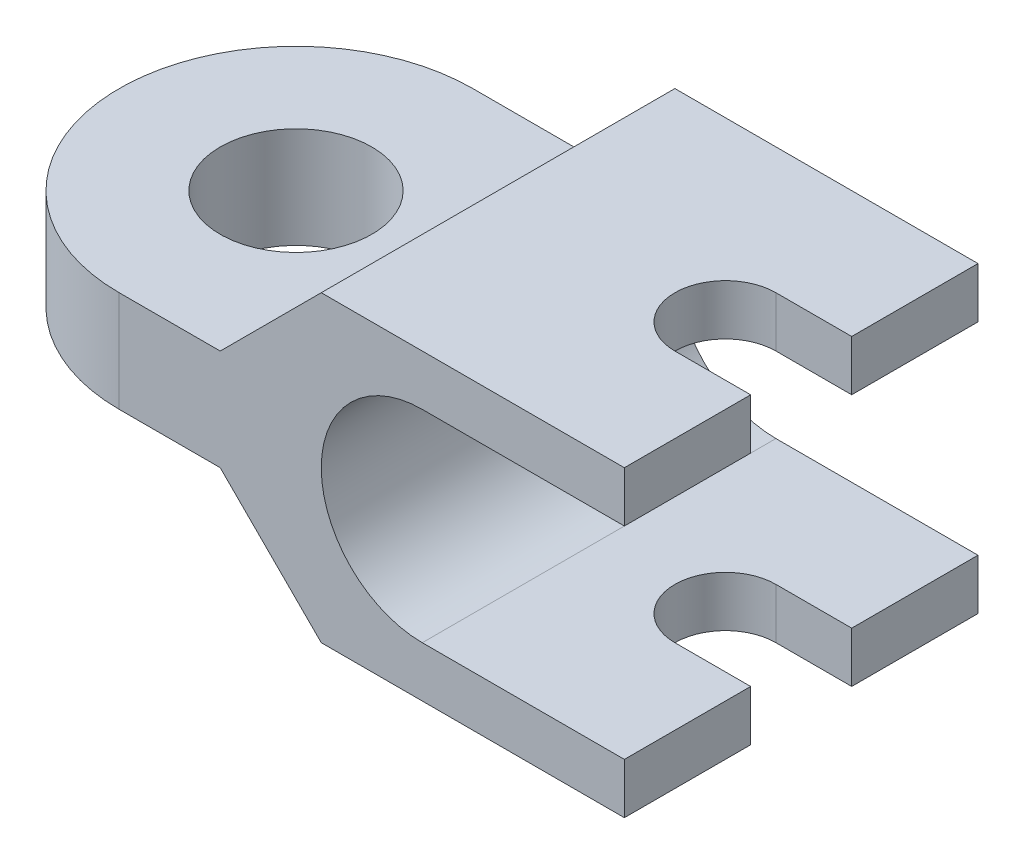
ISO-10303-21;
HEADER;
FILE_DESCRIPTION(('STEP AP214'),'2;1');
FILE_NAME('part.step','',(''),(''),'','','');
FILE_SCHEMA(('AUTOMOTIVE_DESIGN { 1 0 10303 214 1 1 1 1 }'));
ENDSEC;
DATA;
#1=APPLICATION_CONTEXT('core data for automotive mechanical design processes');
#2=APPLICATION_PROTOCOL_DEFINITION('international standard','automotive_design',2000,#1);
#3=PRODUCT_CONTEXT('',#1,'mechanical');
#4=PRODUCT('Part','Part','',(#3));
#5=PRODUCT_RELATED_PRODUCT_CATEGORY('part','',(#4));
#6=PRODUCT_DEFINITION_FORMATION('','',#4);
#7=PRODUCT_DEFINITION_CONTEXT('part definition',#1,'design');
#8=PRODUCT_DEFINITION('design','',#6,#7);
#9=PRODUCT_DEFINITION_SHAPE('','',#8);
#10=(LENGTH_UNIT() NAMED_UNIT(*) SI_UNIT(.MILLI.,.METRE.));
#11=(NAMED_UNIT(*) PLANE_ANGLE_UNIT() SI_UNIT($,.RADIAN.));
#12=(NAMED_UNIT(*) SI_UNIT($,.STERADIAN.) SOLID_ANGLE_UNIT());
#13=UNCERTAINTY_MEASURE_WITH_UNIT(LENGTH_MEASURE(1.E-05),#10,'distance_accuracy_value','');
#14=(GEOMETRIC_REPRESENTATION_CONTEXT(3) GLOBAL_UNCERTAINTY_ASSIGNED_CONTEXT((#13)) GLOBAL_UNIT_ASSIGNED_CONTEXT((#10,
#11,#12)) REPRESENTATION_CONTEXT('',''));
#15=CARTESIAN_POINT('',(0.,0.,0.));
#16=DIRECTION('',(0.,0.,1.));
#17=DIRECTION('',(1.,0.,0.));
#18=AXIS2_PLACEMENT_3D('',#15,#16,#17);
#19=CARTESIAN_POINT('',(-40.,-9.99999999999998,35.));
#20=DIRECTION('',(0.707106781186548,0.707106781186547,0.));
#21=DIRECTION('',(-0.707106781186547,0.707106781186548,0.));
#22=AXIS2_PLACEMENT_3D('',#19,#20,#21);
#23=PLANE('',#22);
#24=DIRECTION('',(-0.707106781186547,0.707106781186548,0.));
#25=VECTOR('',#24,1.);
#26=CARTESIAN_POINT('',(-30.,-20.,15.));
#27=LINE('',#26,#25);
#28=CARTESIAN_POINT('',(-30.,-20.,15.));
#29=VERTEX_POINT('',#28);
#30=CARTESIAN_POINT('',(-40.,-9.99999999999998,15.));
#31=VERTEX_POINT('',#30);
#32=EDGE_CURVE('E239',#29,#31,#27,.T.);
#33=ORIENTED_EDGE('',*,*,#32,.F.);
#34=DIRECTION('',(0.,0.,1.));
#35=VECTOR('',#34,1.);
#36=CARTESIAN_POINT('',(-30.,-20.,-15.));
#37=LINE('',#36,#35);
#38=CARTESIAN_POINT('',(-30.,-20.,-15.));
#39=VERTEX_POINT('',#38);
#40=EDGE_CURVE('E221',#39,#29,#37,.T.);
#41=ORIENTED_EDGE('',*,*,#40,.F.);
#42=DIRECTION('',(-0.707106781186547,0.707106781186548,0.));
#43=VECTOR('',#42,1.);
#44=CARTESIAN_POINT('',(-30.,-20.,-15.));
#45=LINE('',#44,#43);
#46=CARTESIAN_POINT('',(-40.,-9.99999999999998,-15.));
#47=VERTEX_POINT('',#46);
#48=EDGE_CURVE('E60',#39,#47,#45,.T.);
#49=ORIENTED_EDGE('',*,*,#48,.T.);
#50=DIRECTION('',(0.,0.,-1.));
#51=VECTOR('',#50,1.);
#52=CARTESIAN_POINT('',(-40.,-9.99999999999998,35.));
#53=LINE('',#52,#51);
#54=CARTESIAN_POINT('',(-40.,-9.99999999999998,-35.));
#55=VERTEX_POINT('',#54);
#56=EDGE_CURVE('E224',#47,#55,#53,.T.);
#57=ORIENTED_EDGE('',*,*,#56,.T.);
#58=DIRECTION('',(0.707106781186547,-0.707106781186548,0.));
#59=VECTOR('',#58,1.);
#60=CARTESIAN_POINT('',(-40.,-9.99999999999998,-35.));
#61=LINE('',#60,#59);
#62=CARTESIAN_POINT('',(-20.,-30.,-35.));
#63=VERTEX_POINT('',#62);
#64=EDGE_CURVE('E361',#55,#63,#61,.T.);
#65=ORIENTED_EDGE('',*,*,#64,.T.);
#66=DIRECTION('',(0.,0.,-1.));
#67=VECTOR('',#66,1.);
#68=CARTESIAN_POINT('',(-20.,-30.,35.));
#69=LINE('',#68,#67);
#70=CARTESIAN_POINT('',(-20.,-30.,35.));
#71=VERTEX_POINT('',#70);
#72=EDGE_CURVE('E367',#71,#63,#69,.T.);
#73=ORIENTED_EDGE('',*,*,#72,.F.);
#74=DIRECTION('',(0.707106781186547,-0.707106781186548,0.));
#75=VECTOR('',#74,1.);
#76=CARTESIAN_POINT('',(-40.,-9.99999999999998,35.));
#77=LINE('',#76,#75);
#78=CARTESIAN_POINT('',(-40.,-9.99999999999998,35.));
#79=VERTEX_POINT('',#78);
#80=EDGE_CURVE('E338',#79,#71,#77,.T.);
#81=ORIENTED_EDGE('',*,*,#80,.F.);
#82=EDGE_CURVE('E373',#79,#31,#53,.T.);
#83=ORIENTED_EDGE('',*,*,#82,.T.);
#84=EDGE_LOOP('',(#33,#41,#49,#57,#65,#73,#81,#83));
#85=FACE_BOUND('',#84,.T.);
#86=ADVANCED_FACE('F41',(#85),#23,.F.);
#87=CARTESIAN_POINT('',(40.,-30.,35.));
#88=DIRECTION('',(-1.,0.,0.));
#89=DIRECTION('',(0.,0.,1.));
#90=AXIS2_PLACEMENT_3D('',#87,#88,#89);
#91=PLANE('',#90);
#92=DIRECTION('',(0.,1.,0.));
#93=VECTOR('',#92,1.);
#94=CARTESIAN_POINT('',(40.,-30.,-10.));
#95=LINE('',#94,#93);
#96=CARTESIAN_POINT('',(40.,-30.,-10.));
#97=VERTEX_POINT('',#96);
#98=CARTESIAN_POINT('',(40.,-20.,-10.));
#99=VERTEX_POINT('',#98);
#100=EDGE_CURVE('E301',#97,#99,#95,.T.);
#101=ORIENTED_EDGE('',*,*,#100,.F.);
#102=DIRECTION('',(0.,0.,-1.));
#103=VECTOR('',#102,1.);
#104=CARTESIAN_POINT('',(40.,-30.,35.));
#105=LINE('',#104,#103);
#106=CARTESIAN_POINT('',(40.,-30.,-35.));
#107=VERTEX_POINT('',#106);
#108=EDGE_CURVE('E336',#97,#107,#105,.T.);
#109=ORIENTED_EDGE('',*,*,#108,.T.);
#110=DIRECTION('',(0.,1.,0.));
#111=VECTOR('',#110,1.);
#112=CARTESIAN_POINT('',(40.,-30.,-35.));
#113=LINE('',#112,#111);
#114=CARTESIAN_POINT('',(40.,-20.,-35.));
#115=VERTEX_POINT('',#114);
#116=EDGE_CURVE('E314',#107,#115,#113,.T.);
#117=ORIENTED_EDGE('',*,*,#116,.T.);
#118=DIRECTION('',(0.,0.,-1.));
#119=VECTOR('',#118,1.);
#120=CARTESIAN_POINT('',(40.,-20.,35.));
#121=LINE('',#120,#119);
#122=EDGE_CURVE('E400',#99,#115,#121,.T.);
#123=ORIENTED_EDGE('',*,*,#122,.F.);
#124=EDGE_LOOP('',(#101,#109,#117,#123));
#125=FACE_BOUND('',#124,.T.);
#126=ADVANCED_FACE('F500',(#125),#91,.F.);
#127=CARTESIAN_POINT('',(40.,20.,35.));
#128=DIRECTION('',(-1.,0.,0.));
#129=DIRECTION('',(0.,0.,1.));
#130=AXIS2_PLACEMENT_3D('',#127,#128,#129);
#131=PLANE('',#130);
#132=CARTESIAN_POINT('',(40.,20.,-10.));
#133=VERTEX_POINT('',#132);
#134=CARTESIAN_POINT('',(40.,30.,-10.));
#135=VERTEX_POINT('',#134);
#136=EDGE_CURVE('E290',#133,#135,#95,.T.);
#137=ORIENTED_EDGE('',*,*,#136,.F.);
#138=DIRECTION('',(0.,0.,-1.));
#139=VECTOR('',#138,1.);
#140=CARTESIAN_POINT('',(40.,20.,35.));
#141=LINE('',#140,#139);
#142=CARTESIAN_POINT('',(40.,20.,-35.));
#143=VERTEX_POINT('',#142);
#144=EDGE_CURVE('E390',#133,#143,#141,.T.);
#145=ORIENTED_EDGE('',*,*,#144,.T.);
#146=DIRECTION('',(0.,1.,0.));
#147=VECTOR('',#146,1.);
#148=CARTESIAN_POINT('',(40.,20.,-35.));
#149=LINE('',#148,#147);
#150=CARTESIAN_POINT('',(40.,30.,-35.));
#151=VERTEX_POINT('',#150);
#152=EDGE_CURVE('E348',#143,#151,#149,.T.);
#153=ORIENTED_EDGE('',*,*,#152,.T.);
#154=DIRECTION('',(0.,0.,-1.));
#155=VECTOR('',#154,1.);
#156=CARTESIAN_POINT('',(40.,30.,35.));
#157=LINE('',#156,#155);
#158=EDGE_CURVE('E382',#135,#151,#157,.T.);
#159=ORIENTED_EDGE('',*,*,#158,.F.);
#160=EDGE_LOOP('',(#137,#145,#153,#159));
#161=FACE_BOUND('',#160,.T.);
#162=ADVANCED_FACE('F425',(#161),#131,.F.);
#163=CARTESIAN_POINT('',(40.,30.,35.));
#164=DIRECTION('',(0.,-1.,0.));
#165=DIRECTION('',(0.,0.,-1.));
#166=AXIS2_PLACEMENT_3D('',#163,#164,#165);
#167=PLANE('',#166);
#168=DIRECTION('',(-1.,0.,0.));
#169=VECTOR('',#168,1.);
#170=CARTESIAN_POINT('',(40.,30.,-10.));
#171=LINE('',#170,#169);
#172=CARTESIAN_POINT('',(25.,30.,-10.));
#173=VERTEX_POINT('',#172);
#174=EDGE_CURVE('E269',#135,#173,#171,.T.);
#175=ORIENTED_EDGE('',*,*,#174,.F.);
#176=ORIENTED_EDGE('',*,*,#158,.T.);
#177=DIRECTION('',(-1.,0.,0.));
#178=VECTOR('',#177,1.);
#179=CARTESIAN_POINT('',(40.,30.,-35.));
#180=LINE('',#179,#178);
#181=CARTESIAN_POINT('',(-20.,30.,-35.));
#182=VERTEX_POINT('',#181);
#183=EDGE_CURVE('E352',#151,#182,#180,.T.);
#184=ORIENTED_EDGE('',*,*,#183,.T.);
#185=DIRECTION('',(0.,0.,-1.));
#186=VECTOR('',#185,1.);
#187=CARTESIAN_POINT('',(-20.,30.,35.));
#188=LINE('',#187,#186);
#189=CARTESIAN_POINT('',(-20.,30.,35.));
#190=VERTEX_POINT('',#189);
#191=EDGE_CURVE('E379',#190,#182,#188,.T.);
#192=ORIENTED_EDGE('',*,*,#191,.F.);
#193=DIRECTION('',(-1.,0.,0.));
#194=VECTOR('',#193,1.);
#195=CARTESIAN_POINT('',(40.,30.,35.));
#196=LINE('',#195,#194);
#197=CARTESIAN_POINT('',(40.,30.,35.));
#198=VERTEX_POINT('',#197);
#199=EDGE_CURVE('E330',#198,#190,#196,.T.);
#200=ORIENTED_EDGE('',*,*,#199,.F.);
#201=CARTESIAN_POINT('',(40.,30.,10.));
#202=VERTEX_POINT('',#201);
#203=EDGE_CURVE('E383',#198,#202,#157,.T.);
#204=ORIENTED_EDGE('',*,*,#203,.T.);
#205=DIRECTION('',(1.,0.,0.));
#206=VECTOR('',#205,1.);
#207=CARTESIAN_POINT('',(25.,30.,10.));
#208=LINE('',#207,#206);
#209=CARTESIAN_POINT('',(25.,30.,9.99999999999999));
#210=VERTEX_POINT('',#209);
#211=EDGE_CURVE('E277',#210,#202,#208,.T.);
#212=ORIENTED_EDGE('',*,*,#211,.F.);
#213=CARTESIAN_POINT('',(25.,30.,0.));
#214=DIRECTION('',(0.,1.,0.));
#215=DIRECTION('',(0.,0.,1.));
#216=AXIS2_PLACEMENT_3D('',#213,#214,#215);
#217=CIRCLE('',#216,10.);
#218=EDGE_CURVE('E272',#173,#210,#217,.T.);
#219=ORIENTED_EDGE('',*,*,#218,.F.);
#220=EDGE_LOOP('',(#175,#176,#184,#192,#200,#204,#212,#219));
#221=FACE_BOUND('',#220,.T.);
#222=ADVANCED_FACE('F426',(#221),#167,.F.);
#223=CARTESIAN_POINT('',(-60.,9.99999999999998,0.));
#224=DIRECTION('',(0.,-1.,0.));
#225=DIRECTION('',(0.,0.,-1.));
#226=AXIS2_PLACEMENT_3D('',#223,#224,#225);
#227=CYLINDRICAL_SURFACE('',#226,35.);
#228=DIRECTION('',(0.,-1.,0.));
#229=VECTOR('',#228,1.);
#230=CARTESIAN_POINT('',(-60.,0.,35.));
#231=LINE('',#230,#229);
#232=CARTESIAN_POINT('',(-60.,9.99999999999998,35.));
#233=VERTEX_POINT('',#232);
#234=CARTESIAN_POINT('',(-60.,-9.99999999999998,35.));
#235=VERTEX_POINT('',#234);
#236=EDGE_CURVE('E402',#233,#235,#231,.T.);
#237=ORIENTED_EDGE('',*,*,#236,.F.);
#238=CARTESIAN_POINT('',(-60.,9.99999999999998,0.));
#239=DIRECTION('',(0.,-1.,0.));
#240=DIRECTION('',(1.,0.,0.));
#241=AXIS2_PLACEMENT_3D('',#238,#239,#240);
#242=CIRCLE('',#241,35.);
#243=CARTESIAN_POINT('',(-60.,9.99999999999998,-35.));
#244=VERTEX_POINT('',#243);
#245=EDGE_CURVE('E409',#244,#233,#242,.F.);
#246=ORIENTED_EDGE('',*,*,#245,.F.);
#247=DIRECTION('',(0.,1.,0.));
#248=VECTOR('',#247,1.);
#249=CARTESIAN_POINT('',(-60.,9.99999999999998,-35.));
#250=LINE('',#249,#248);
#251=CARTESIAN_POINT('',(-60.,-9.99999999999998,-35.));
#252=VERTEX_POINT('',#251);
#253=EDGE_CURVE('E404',#252,#244,#250,.T.);
#254=ORIENTED_EDGE('',*,*,#253,.F.);
#255=CARTESIAN_POINT('',(-60.,-9.99999999999998,0.));
#256=DIRECTION('',(0.,1.,0.));
#257=DIRECTION('',(-1.,0.,0.));
#258=AXIS2_PLACEMENT_3D('',#255,#256,#257);
#259=CIRCLE('',#258,35.);
#260=EDGE_CURVE('E410',#235,#252,#259,.F.);
#261=ORIENTED_EDGE('',*,*,#260,.F.);
#262=EDGE_LOOP('',(#237,#246,#254,#261));
#263=FACE_BOUND('',#262,.T.);
#264=ADVANCED_FACE('F42',(#263),#227,.T.);
#265=CARTESIAN_POINT('',(40.,-30.,35.));
#266=VERTEX_POINT('',#265);
#267=CARTESIAN_POINT('',(40.,-30.,10.));
#268=VERTEX_POINT('',#267);
#269=EDGE_CURVE('E370',#266,#268,#105,.T.);
#270=ORIENTED_EDGE('',*,*,#269,.T.);
#271=DIRECTION('',(0.,1.,0.));
#272=VECTOR('',#271,1.);
#273=CARTESIAN_POINT('',(40.,-30.,10.));
#274=LINE('',#273,#272);
#275=CARTESIAN_POINT('',(40.,-20.,10.));
#276=VERTEX_POINT('',#275);
#277=EDGE_CURVE('E287',#268,#276,#274,.T.);
#278=ORIENTED_EDGE('',*,*,#277,.T.);
#279=CARTESIAN_POINT('',(40.,-20.,35.));
#280=VERTEX_POINT('',#279);
#281=EDGE_CURVE('E397',#280,#276,#121,.T.);
#282=ORIENTED_EDGE('',*,*,#281,.F.);
#283=DIRECTION('',(0.,1.,0.));
#284=VECTOR('',#283,1.);
#285=CARTESIAN_POINT('',(40.,-30.,35.));
#286=LINE('',#285,#284);
#287=EDGE_CURVE('E312',#266,#280,#286,.T.);
#288=ORIENTED_EDGE('',*,*,#287,.F.);
#289=EDGE_LOOP('',(#270,#278,#282,#288));
#290=FACE_BOUND('',#289,.T.);
#291=ADVANCED_FACE('F485',(#290),#91,.F.);
#292=CARTESIAN_POINT('',(40.,-20.,35.));
#293=DIRECTION('',(0.,-1.,0.));
#294=DIRECTION('',(1.,0.,0.));
#295=AXIS2_PLACEMENT_3D('',#292,#293,#294);
#296=PLANE('',#295);
#297=ORIENTED_EDGE('',*,*,#281,.T.);
#298=DIRECTION('',(-1.,0.,0.));
#299=VECTOR('',#298,1.);
#300=CARTESIAN_POINT('',(40.,-20.,10.));
#301=LINE('',#300,#299);
#302=CARTESIAN_POINT('',(25.,-20.,9.99999999999999));
#303=VERTEX_POINT('',#302);
#304=EDGE_CURVE('E313',#276,#303,#301,.T.);
#305=ORIENTED_EDGE('',*,*,#304,.T.);
#306=CARTESIAN_POINT('',(25.,-20.,0.));
#307=DIRECTION('',(0.,-1.,0.));
#308=DIRECTION('',(1.,0.,0.));
#309=AXIS2_PLACEMENT_3D('',#306,#307,#308);
#310=CIRCLE('',#309,10.);
#311=CARTESIAN_POINT('',(25.,-20.,-10.));
#312=VERTEX_POINT('',#311);
#313=EDGE_CURVE('E304',#303,#312,#310,.T.);
#314=ORIENTED_EDGE('',*,*,#313,.T.);
#315=DIRECTION('',(1.,0.,0.));
#316=VECTOR('',#315,1.);
#317=CARTESIAN_POINT('',(40.,-20.,-10.));
#318=LINE('',#317,#316);
#319=EDGE_CURVE('E306',#312,#99,#318,.T.);
#320=ORIENTED_EDGE('',*,*,#319,.T.);
#321=ORIENTED_EDGE('',*,*,#122,.T.);
#322=DIRECTION('',(-1.,0.,0.));
#323=VECTOR('',#322,1.);
#324=CARTESIAN_POINT('',(40.,-20.,-35.));
#325=LINE('',#324,#323);
#326=CARTESIAN_POINT('',(0.,-20.,-35.));
#327=VERTEX_POINT('',#326);
#328=EDGE_CURVE('E342',#115,#327,#325,.T.);
#329=ORIENTED_EDGE('',*,*,#328,.T.);
#330=DIRECTION('',(0.,0.,-1.));
#331=VECTOR('',#330,1.);
#332=CARTESIAN_POINT('',(0.,-20.,35.));
#333=LINE('',#332,#331);
#334=CARTESIAN_POINT('',(0.,-20.,35.));
#335=VERTEX_POINT('',#334);
#336=EDGE_CURVE('E395',#335,#327,#333,.T.);
#337=ORIENTED_EDGE('',*,*,#336,.F.);
#338=DIRECTION('',(-1.,0.,0.));
#339=VECTOR('',#338,1.);
#340=CARTESIAN_POINT('',(40.,-20.,35.));
#341=LINE('',#340,#339);
#342=EDGE_CURVE('E318',#280,#335,#341,.T.);
#343=ORIENTED_EDGE('',*,*,#342,.F.);
#344=EDGE_LOOP('',(#297,#305,#314,#320,#321,#329,#337,#343));
#345=FACE_BOUND('',#344,.T.);
#346=ADVANCED_FACE('F484',(#345),#296,.F.);
#347=CARTESIAN_POINT('',(0.,0.,35.));
#348=DIRECTION('',(0.,0.,-1.));
#349=DIRECTION('',(-1.,0.,0.));
#350=AXIS2_PLACEMENT_3D('',#347,#348,#349);
#351=CYLINDRICAL_SURFACE('',#350,20.);
#352=CARTESIAN_POINT('',(0.,0.,-35.));
#353=DIRECTION('',(0.,0.,-1.));
#354=DIRECTION('',(-1.,0.,0.));
#355=AXIS2_PLACEMENT_3D('',#352,#353,#354);
#356=CIRCLE('',#355,20.);
#357=CARTESIAN_POINT('',(0.,20.,-35.));
#358=VERTEX_POINT('',#357);
#359=EDGE_CURVE('E344',#327,#358,#356,.T.);
#360=ORIENTED_EDGE('',*,*,#359,.T.);
#361=DIRECTION('',(0.,0.,-1.));
#362=VECTOR('',#361,1.);
#363=CARTESIAN_POINT('',(0.,20.,35.));
#364=LINE('',#363,#362);
#365=CARTESIAN_POINT('',(0.,20.,35.));
#366=VERTEX_POINT('',#365);
#367=EDGE_CURVE('E393',#366,#358,#364,.T.);
#368=ORIENTED_EDGE('',*,*,#367,.F.);
#369=CARTESIAN_POINT('',(0.,0.,35.));
#370=DIRECTION('',(0.,0.,-1.));
#371=DIRECTION('',(-1.,0.,0.));
#372=AXIS2_PLACEMENT_3D('',#369,#370,#371);
#373=CIRCLE('',#372,20.);
#374=EDGE_CURVE('E321',#335,#366,#373,.T.);
#375=ORIENTED_EDGE('',*,*,#374,.F.);
#376=ORIENTED_EDGE('',*,*,#336,.T.);
#377=EDGE_LOOP('',(#360,#368,#375,#376));
#378=FACE_BOUND('',#377,.T.);
#379=ADVANCED_FACE('F486',(#378),#351,.F.);
#380=CARTESIAN_POINT('',(0.,20.,35.));
#381=DIRECTION('',(0.,1.,0.));
#382=DIRECTION('',(-1.,0.,0.));
#383=AXIS2_PLACEMENT_3D('',#380,#381,#382);
#384=PLANE('',#383);
#385=CARTESIAN_POINT('',(25.,20.,0.));
#386=DIRECTION('',(0.,1.,0.));
#387=DIRECTION('',(-1.,0.,0.));
#388=AXIS2_PLACEMENT_3D('',#385,#386,#387);
#389=CIRCLE('',#388,10.);
#390=CARTESIAN_POINT('',(25.,20.,-10.));
#391=VERTEX_POINT('',#390);
#392=CARTESIAN_POINT('',(25.,20.,9.99999999999999));
#393=VERTEX_POINT('',#392);
#394=EDGE_CURVE('E292',#391,#393,#389,.T.);
#395=ORIENTED_EDGE('',*,*,#394,.T.);
#396=DIRECTION('',(1.,0.,0.));
#397=VECTOR('',#396,1.);
#398=CARTESIAN_POINT('',(0.,20.,10.));
#399=LINE('',#398,#397);
#400=CARTESIAN_POINT('',(40.,20.,10.));
#401=VERTEX_POINT('',#400);
#402=EDGE_CURVE('E11',#393,#401,#399,.T.);
#403=ORIENTED_EDGE('',*,*,#402,.T.);
#404=CARTESIAN_POINT('',(40.,20.,35.));
#405=VERTEX_POINT('',#404);
#406=EDGE_CURVE('E389',#405,#401,#141,.T.);
#407=ORIENTED_EDGE('',*,*,#406,.F.);
#408=DIRECTION('',(1.,0.,0.));
#409=VECTOR('',#408,1.);
#410=CARTESIAN_POINT('',(0.,20.,35.));
#411=LINE('',#410,#409);
#412=EDGE_CURVE('E323',#366,#405,#411,.T.);
#413=ORIENTED_EDGE('',*,*,#412,.F.);
#414=ORIENTED_EDGE('',*,*,#367,.T.);
#415=DIRECTION('',(1.,0.,0.));
#416=VECTOR('',#415,1.);
#417=CARTESIAN_POINT('',(0.,20.,-35.));
#418=LINE('',#417,#416);
#419=EDGE_CURVE('E350',#358,#143,#418,.T.);
#420=ORIENTED_EDGE('',*,*,#419,.T.);
#421=ORIENTED_EDGE('',*,*,#144,.F.);
#422=DIRECTION('',(-1.,0.,0.));
#423=VECTOR('',#422,1.);
#424=CARTESIAN_POINT('',(0.,20.,-9.99999999999999));
#425=LINE('',#424,#423);
#426=EDGE_CURVE('E49',#133,#391,#425,.T.);
#427=ORIENTED_EDGE('',*,*,#426,.T.);
#428=EDGE_LOOP('',(#395,#403,#407,#413,#414,#420,#421,#427));
#429=FACE_BOUND('',#428,.T.);
#430=ADVANCED_FACE('F412',(#429),#384,.F.);
#431=ORIENTED_EDGE('',*,*,#406,.T.);
#432=EDGE_CURVE('E295',#401,#202,#274,.T.);
#433=ORIENTED_EDGE('',*,*,#432,.T.);
#434=ORIENTED_EDGE('',*,*,#203,.F.);
#435=DIRECTION('',(0.,1.,0.));
#436=VECTOR('',#435,1.);
#437=CARTESIAN_POINT('',(40.,20.,35.));
#438=LINE('',#437,#436);
#439=EDGE_CURVE('E324',#405,#198,#438,.T.);
#440=ORIENTED_EDGE('',*,*,#439,.F.);
#441=EDGE_LOOP('',(#431,#433,#434,#440));
#442=FACE_BOUND('',#441,.T.);
#443=ADVANCED_FACE('F439',(#442),#131,.F.);
#444=CARTESIAN_POINT('',(-20.,30.,35.));
#445=DIRECTION('',(0.707106781186548,-0.707106781186547,0.));
#446=DIRECTION('',(0.707106781186547,0.707106781186548,0.));
#447=AXIS2_PLACEMENT_3D('',#444,#445,#446);
#448=PLANE('',#447);
#449=DIRECTION('',(0.,0.,1.));
#450=VECTOR('',#449,1.);
#451=CARTESIAN_POINT('',(-30.,20.,-15.));
#452=LINE('',#451,#450);
#453=CARTESIAN_POINT('',(-30.,20.,-15.));
#454=VERTEX_POINT('',#453);
#455=CARTESIAN_POINT('',(-30.,20.,15.));
#456=VERTEX_POINT('',#455);
#457=EDGE_CURVE('E270',#454,#456,#452,.T.);
#458=ORIENTED_EDGE('',*,*,#457,.T.);
#459=DIRECTION('',(-0.707106781186547,-0.707106781186548,0.));
#460=VECTOR('',#459,1.);
#461=CARTESIAN_POINT('',(-30.,20.,15.));
#462=LINE('',#461,#460);
#463=CARTESIAN_POINT('',(-40.,9.99999999999998,15.));
#464=VERTEX_POINT('',#463);
#465=EDGE_CURVE('E249',#456,#464,#462,.T.);
#466=ORIENTED_EDGE('',*,*,#465,.T.);
#467=DIRECTION('',(0.,0.,-1.));
#468=VECTOR('',#467,1.);
#469=CARTESIAN_POINT('',(-40.,9.99999999999998,35.));
#470=LINE('',#469,#468);
#471=CARTESIAN_POINT('',(-40.,9.99999999999998,35.));
#472=VERTEX_POINT('',#471);
#473=EDGE_CURVE('E380',#472,#464,#470,.T.);
#474=ORIENTED_EDGE('',*,*,#473,.F.);
#475=DIRECTION('',(-0.707106781186547,-0.707106781186548,0.));
#476=VECTOR('',#475,1.);
#477=CARTESIAN_POINT('',(-20.,30.,35.));
#478=LINE('',#477,#476);
#479=EDGE_CURVE('E328',#190,#472,#478,.T.);
#480=ORIENTED_EDGE('',*,*,#479,.F.);
#481=ORIENTED_EDGE('',*,*,#191,.T.);
#482=DIRECTION('',(-0.707106781186547,-0.707106781186548,0.));
#483=VECTOR('',#482,1.);
#484=CARTESIAN_POINT('',(-20.,30.,-35.));
#485=LINE('',#484,#483);
#486=CARTESIAN_POINT('',(-40.,9.99999999999998,-35.));
#487=VERTEX_POINT('',#486);
#488=EDGE_CURVE('E351',#182,#487,#485,.T.);
#489=ORIENTED_EDGE('',*,*,#488,.T.);
#490=CARTESIAN_POINT('',(-40.,9.99999999999998,-15.));
#491=VERTEX_POINT('',#490);
#492=EDGE_CURVE('E376',#491,#487,#470,.T.);
#493=ORIENTED_EDGE('',*,*,#492,.F.);
#494=DIRECTION('',(-0.707106781186547,-0.707106781186548,0.));
#495=VECTOR('',#494,1.);
#496=CARTESIAN_POINT('',(-30.,20.,-15.));
#497=LINE('',#496,#495);
#498=EDGE_CURVE('E253',#454,#491,#497,.T.);
#499=ORIENTED_EDGE('',*,*,#498,.F.);
#500=EDGE_LOOP('',(#458,#466,#474,#480,#481,#489,#493,#499));
#501=FACE_BOUND('',#500,.T.);
#502=ADVANCED_FACE('F456',(#501),#448,.F.);
#503=CARTESIAN_POINT('',(-40.,9.99999999999998,35.));
#504=DIRECTION('',(0.,-1.,0.));
#505=DIRECTION('',(1.,0.,0.));
#506=AXIS2_PLACEMENT_3D('',#503,#504,#505);
#507=PLANE('',#506);
#508=CARTESIAN_POINT('',(-60.,9.99999999999998,0.));
#509=DIRECTION('',(0.,1.,0.));
#510=DIRECTION('',(-1.,0.,0.));
#511=AXIS2_PLACEMENT_3D('',#508,#509,#510);
#512=CIRCLE('',#511,15.);
#513=CARTESIAN_POINT('',(-75.,9.99999999999998,0.));
#514=VERTEX_POINT('',#513);
#515=EDGE_CURVE('E235',#514,#514,#512,.T.);
#516=ORIENTED_EDGE('',*,*,#515,.F.);
#517=EDGE_LOOP('',(#516));
#518=FACE_BOUND('',#517,.T.);
#519=DIRECTION('',(-1.,0.,0.));
#520=VECTOR('',#519,1.);
#521=CARTESIAN_POINT('',(-40.,9.99999999999998,-35.));
#522=LINE('',#521,#520);
#523=EDGE_CURVE('E357',#487,#244,#522,.T.);
#524=ORIENTED_EDGE('',*,*,#523,.T.);
#525=ORIENTED_EDGE('',*,*,#245,.T.);
#526=DIRECTION('',(-1.,0.,0.));
#527=VECTOR('',#526,1.);
#528=CARTESIAN_POINT('',(-40.,9.99999999999998,35.));
#529=LINE('',#528,#527);
#530=EDGE_CURVE('E332',#472,#233,#529,.T.);
#531=ORIENTED_EDGE('',*,*,#530,.F.);
#532=ORIENTED_EDGE('',*,*,#473,.T.);
#533=DIRECTION('',(1.,0.,0.));
#534=VECTOR('',#533,1.);
#535=CARTESIAN_POINT('',(-40.,9.99999999999998,15.));
#536=LINE('',#535,#534);
#537=CARTESIAN_POINT('',(-30.,9.99999999999998,15.));
#538=VERTEX_POINT('',#537);
#539=EDGE_CURVE('E263',#464,#538,#536,.T.);
#540=ORIENTED_EDGE('',*,*,#539,.T.);
#541=DIRECTION('',(0.,0.,1.));
#542=VECTOR('',#541,1.);
#543=CARTESIAN_POINT('',(-30.,9.99999999999998,-15.));
#544=LINE('',#543,#542);
#545=CARTESIAN_POINT('',(-30.,9.99999999999998,-15.));
#546=VERTEX_POINT('',#545);
#547=EDGE_CURVE('E257',#546,#538,#544,.T.);
#548=ORIENTED_EDGE('',*,*,#547,.F.);
#549=DIRECTION('',(1.,0.,0.));
#550=VECTOR('',#549,1.);
#551=CARTESIAN_POINT('',(-40.,9.99999999999998,-15.));
#552=LINE('',#551,#550);
#553=EDGE_CURVE('E255',#491,#546,#552,.T.);
#554=ORIENTED_EDGE('',*,*,#553,.F.);
#555=ORIENTED_EDGE('',*,*,#492,.T.);
#556=EDGE_LOOP('',(#524,#525,#531,#532,#540,#548,#554,#555));
#557=FACE_BOUND('',#556,.T.);
#558=ADVANCED_FACE('F461',(#518,#557),#507,.F.);
#559=CARTESIAN_POINT('',(-95.,-9.99999999999998,35.));
#560=DIRECTION('',(0.,1.,0.));
#561=DIRECTION('',(-1.,0.,0.));
#562=AXIS2_PLACEMENT_3D('',#559,#560,#561);
#563=PLANE('',#562);
#564=CARTESIAN_POINT('',(-60.,-9.99999999999998,0.));
#565=DIRECTION('',(0.,1.,0.));
#566=DIRECTION('',(-1.,0.,0.));
#567=AXIS2_PLACEMENT_3D('',#564,#565,#566);
#568=CIRCLE('',#567,15.);
#569=CARTESIAN_POINT('',(-75.,-9.99999999999998,0.));
#570=VERTEX_POINT('',#569);
#571=EDGE_CURVE('E250',#570,#570,#568,.F.);
#572=ORIENTED_EDGE('',*,*,#571,.F.);
#573=EDGE_LOOP('',(#572));
#574=FACE_BOUND('',#573,.T.);
#575=DIRECTION('',(1.,0.,0.));
#576=VECTOR('',#575,1.);
#577=CARTESIAN_POINT('',(-95.,-9.99999999999998,35.));
#578=LINE('',#577,#576);
#579=EDGE_CURVE('E331',#235,#79,#578,.T.);
#580=ORIENTED_EDGE('',*,*,#579,.F.);
#581=ORIENTED_EDGE('',*,*,#260,.T.);
#582=DIRECTION('',(1.,0.,0.));
#583=VECTOR('',#582,1.);
#584=CARTESIAN_POINT('',(-95.,-9.99999999999998,-35.));
#585=LINE('',#584,#583);
#586=EDGE_CURVE('E363',#252,#55,#585,.T.);
#587=ORIENTED_EDGE('',*,*,#586,.T.);
#588=ORIENTED_EDGE('',*,*,#56,.F.);
#589=DIRECTION('',(1.,0.,0.));
#590=VECTOR('',#589,1.);
#591=CARTESIAN_POINT('',(-40.,-9.99999999999998,-15.));
#592=LINE('',#591,#590);
#593=CARTESIAN_POINT('',(-30.,-9.99999999999998,-15.));
#594=VERTEX_POINT('',#593);
#595=EDGE_CURVE('E216',#47,#594,#592,.T.);
#596=ORIENTED_EDGE('',*,*,#595,.T.);
#597=DIRECTION('',(0.,0.,1.));
#598=VECTOR('',#597,1.);
#599=CARTESIAN_POINT('',(-30.,-9.99999999999998,-15.));
#600=LINE('',#599,#598);
#601=CARTESIAN_POINT('',(-30.,-9.99999999999998,15.));
#602=VERTEX_POINT('',#601);
#603=EDGE_CURVE('E219',#594,#602,#600,.T.);
#604=ORIENTED_EDGE('',*,*,#603,.T.);
#605=DIRECTION('',(1.,0.,0.));
#606=VECTOR('',#605,1.);
#607=CARTESIAN_POINT('',(-40.,-9.99999999999998,15.));
#608=LINE('',#607,#606);
#609=EDGE_CURVE('E237',#31,#602,#608,.T.);
#610=ORIENTED_EDGE('',*,*,#609,.F.);
#611=ORIENTED_EDGE('',*,*,#82,.F.);
#612=EDGE_LOOP('',(#580,#581,#587,#588,#596,#604,#610,#611));
#613=FACE_BOUND('',#612,.T.);
#614=ADVANCED_FACE('F218',(#574,#613),#563,.F.);
#615=CARTESIAN_POINT('',(-20.,-30.,35.));
#616=DIRECTION('',(0.,1.,0.));
#617=DIRECTION('',(0.,0.,1.));
#618=AXIS2_PLACEMENT_3D('',#615,#616,#617);
#619=PLANE('',#618);
#620=CARTESIAN_POINT('',(25.,-30.,0.));
#621=DIRECTION('',(0.,1.,0.));
#622=DIRECTION('',(0.,0.,1.));
#623=AXIS2_PLACEMENT_3D('',#620,#621,#622);
#624=CIRCLE('',#623,10.);
#625=CARTESIAN_POINT('',(25.,-30.,-10.));
#626=VERTEX_POINT('',#625);
#627=CARTESIAN_POINT('',(25.,-30.,9.99999999999999));
#628=VERTEX_POINT('',#627);
#629=EDGE_CURVE('E283',#626,#628,#624,.T.);
#630=ORIENTED_EDGE('',*,*,#629,.T.);
#631=DIRECTION('',(1.,0.,0.));
#632=VECTOR('',#631,1.);
#633=CARTESIAN_POINT('',(25.,-30.,10.));
#634=LINE('',#633,#632);
#635=EDGE_CURVE('E285',#628,#268,#634,.T.);
#636=ORIENTED_EDGE('',*,*,#635,.T.);
#637=ORIENTED_EDGE('',*,*,#269,.F.);
#638=DIRECTION('',(1.,0.,0.));
#639=VECTOR('',#638,1.);
#640=CARTESIAN_POINT('',(-20.,-30.,35.));
#641=LINE('',#640,#639);
#642=EDGE_CURVE('E337',#71,#266,#641,.T.);
#643=ORIENTED_EDGE('',*,*,#642,.F.);
#644=ORIENTED_EDGE('',*,*,#72,.T.);
#645=DIRECTION('',(1.,0.,0.));
#646=VECTOR('',#645,1.);
#647=CARTESIAN_POINT('',(-20.,-30.,-35.));
#648=LINE('',#647,#646);
#649=EDGE_CURVE('E317',#63,#107,#648,.T.);
#650=ORIENTED_EDGE('',*,*,#649,.T.);
#651=ORIENTED_EDGE('',*,*,#108,.F.);
#652=DIRECTION('',(-1.,0.,0.));
#653=VECTOR('',#652,1.);
#654=CARTESIAN_POINT('',(40.,-30.,-10.));
#655=LINE('',#654,#653);
#656=EDGE_CURVE('E279',#97,#626,#655,.T.);
#657=ORIENTED_EDGE('',*,*,#656,.T.);
#658=EDGE_LOOP('',(#630,#636,#637,#643,#644,#650,#651,#657));
#659=FACE_BOUND('',#658,.T.);
#660=ADVANCED_FACE('F476',(#659),#619,.F.);
#661=CARTESIAN_POINT('',(0.,0.,35.));
#662=DIRECTION('',(0.,0.,-1.));
#663=DIRECTION('',(-1.,0.,0.));
#664=AXIS2_PLACEMENT_3D('',#661,#662,#663);
#665=PLANE('',#664);
#666=ORIENTED_EDGE('',*,*,#530,.T.);
#667=ORIENTED_EDGE('',*,*,#236,.T.);
#668=ORIENTED_EDGE('',*,*,#579,.T.);
#669=ORIENTED_EDGE('',*,*,#80,.T.);
#670=ORIENTED_EDGE('',*,*,#642,.T.);
#671=ORIENTED_EDGE('',*,*,#287,.T.);
#672=ORIENTED_EDGE('',*,*,#342,.T.);
#673=ORIENTED_EDGE('',*,*,#374,.T.);
#674=ORIENTED_EDGE('',*,*,#412,.T.);
#675=ORIENTED_EDGE('',*,*,#439,.T.);
#676=ORIENTED_EDGE('',*,*,#199,.T.);
#677=ORIENTED_EDGE('',*,*,#479,.T.);
#678=EDGE_LOOP('',(#666,#667,#668,#669,#670,#671,#672,#673,#674,#675,#676,#677));
#679=FACE_BOUND('',#678,.T.);
#680=ADVANCED_FACE('F441',(#679),#665,.F.);
#681=CARTESIAN_POINT('',(0.,0.,-35.));
#682=DIRECTION('',(0.,0.,-1.));
#683=DIRECTION('',(-1.,0.,0.));
#684=AXIS2_PLACEMENT_3D('',#681,#682,#683);
#685=PLANE('',#684);
#686=ORIENTED_EDGE('',*,*,#586,.F.);
#687=ORIENTED_EDGE('',*,*,#253,.T.);
#688=ORIENTED_EDGE('',*,*,#523,.F.);
#689=ORIENTED_EDGE('',*,*,#488,.F.);
#690=ORIENTED_EDGE('',*,*,#183,.F.);
#691=ORIENTED_EDGE('',*,*,#152,.F.);
#692=ORIENTED_EDGE('',*,*,#419,.F.);
#693=ORIENTED_EDGE('',*,*,#359,.F.);
#694=ORIENTED_EDGE('',*,*,#328,.F.);
#695=ORIENTED_EDGE('',*,*,#116,.F.);
#696=ORIENTED_EDGE('',*,*,#649,.F.);
#697=ORIENTED_EDGE('',*,*,#64,.F.);
#698=EDGE_LOOP('',(#686,#687,#688,#689,#690,#691,#692,#693,#694,#695,#696,#697));
#699=FACE_BOUND('',#698,.T.);
#700=ADVANCED_FACE('F455',(#699),#685,.T.);
#701=CARTESIAN_POINT('',(25.,-30.,0.));
#702=DIRECTION('',(0.,1.,0.));
#703=DIRECTION('',(0.,0.,1.));
#704=AXIS2_PLACEMENT_3D('',#701,#702,#703);
#705=CYLINDRICAL_SURFACE('',#704,10.);
#706=DIRECTION('',(0.,1.,0.));
#707=VECTOR('',#706,1.);
#708=CARTESIAN_POINT('',(25.,-30.,9.99999999999999));
#709=LINE('',#708,#707);
#710=EDGE_CURVE('E291',#628,#303,#709,.T.);
#711=ORIENTED_EDGE('',*,*,#710,.F.);
#712=ORIENTED_EDGE('',*,*,#629,.F.);
#713=DIRECTION('',(0.,1.,0.));
#714=VECTOR('',#713,1.);
#715=CARTESIAN_POINT('',(25.,-30.,-10.));
#716=LINE('',#715,#714);
#717=EDGE_CURVE('E299',#626,#312,#716,.T.);
#718=ORIENTED_EDGE('',*,*,#717,.T.);
#719=ORIENTED_EDGE('',*,*,#313,.F.);
#720=EDGE_LOOP('',(#711,#712,#718,#719));
#721=FACE_BOUND('',#720,.T.);
#722=ADVANCED_FACE('F607',(#721),#705,.F.);
#723=CARTESIAN_POINT('',(40.,-30.,-10.));
#724=DIRECTION('',(0.,0.,-1.));
#725=DIRECTION('',(-1.,0.,0.));
#726=AXIS2_PLACEMENT_3D('',#723,#724,#725);
#727=PLANE('',#726);
#728=ORIENTED_EDGE('',*,*,#717,.F.);
#729=ORIENTED_EDGE('',*,*,#656,.F.);
#730=ORIENTED_EDGE('',*,*,#100,.T.);
#731=ORIENTED_EDGE('',*,*,#319,.F.);
#732=EDGE_LOOP('',(#728,#729,#730,#731));
#733=FACE_BOUND('',#732,.T.);
#734=ADVANCED_FACE('F615',(#733),#727,.F.);
#735=CARTESIAN_POINT('',(25.,-30.,10.));
#736=DIRECTION('',(0.,0.,1.));
#737=DIRECTION('',(1.,0.,0.));
#738=AXIS2_PLACEMENT_3D('',#735,#736,#737);
#739=PLANE('',#738);
#740=ORIENTED_EDGE('',*,*,#277,.F.);
#741=ORIENTED_EDGE('',*,*,#635,.F.);
#742=ORIENTED_EDGE('',*,*,#710,.T.);
#743=ORIENTED_EDGE('',*,*,#304,.F.);
#744=EDGE_LOOP('',(#740,#741,#742,#743));
#745=FACE_BOUND('',#744,.T.);
#746=ADVANCED_FACE('F618',(#745),#739,.F.);
#747=EDGE_CURVE('E298',#393,#210,#709,.T.);
#748=ORIENTED_EDGE('',*,*,#747,.T.);
#749=ORIENTED_EDGE('',*,*,#211,.T.);
#750=ORIENTED_EDGE('',*,*,#432,.F.);
#751=ORIENTED_EDGE('',*,*,#402,.F.);
#752=EDGE_LOOP('',(#748,#749,#750,#751));
#753=FACE_BOUND('',#752,.T.);
#754=ADVANCED_FACE('F432',(#753),#739,.F.);
#755=ORIENTED_EDGE('',*,*,#136,.T.);
#756=ORIENTED_EDGE('',*,*,#174,.T.);
#757=EDGE_CURVE('E296',#391,#173,#716,.T.);
#758=ORIENTED_EDGE('',*,*,#757,.F.);
#759=ORIENTED_EDGE('',*,*,#426,.F.);
#760=EDGE_LOOP('',(#755,#756,#758,#759));
#761=FACE_BOUND('',#760,.T.);
#762=ADVANCED_FACE('F417',(#761),#727,.F.);
#763=ORIENTED_EDGE('',*,*,#757,.T.);
#764=ORIENTED_EDGE('',*,*,#218,.T.);
#765=ORIENTED_EDGE('',*,*,#747,.F.);
#766=ORIENTED_EDGE('',*,*,#394,.F.);
#767=EDGE_LOOP('',(#763,#764,#765,#766));
#768=FACE_BOUND('',#767,.T.);
#769=ADVANCED_FACE('F431',(#768),#705,.F.);
#770=CARTESIAN_POINT('',(-30.,9.99999999999998,-15.));
#771=DIRECTION('',(1.,0.,0.));
#772=DIRECTION('',(0.,0.,-1.));
#773=AXIS2_PLACEMENT_3D('',#770,#771,#772);
#774=PLANE('',#773);
#775=DIRECTION('',(0.,1.,0.));
#776=VECTOR('',#775,1.);
#777=CARTESIAN_POINT('',(-30.,9.99999999999998,15.));
#778=LINE('',#777,#776);
#779=EDGE_CURVE('E61',#538,#456,#778,.T.);
#780=ORIENTED_EDGE('',*,*,#779,.T.);
#781=ORIENTED_EDGE('',*,*,#457,.F.);
#782=DIRECTION('',(0.,1.,0.));
#783=VECTOR('',#782,1.);
#784=CARTESIAN_POINT('',(-30.,9.99999999999998,-15.));
#785=LINE('',#784,#783);
#786=EDGE_CURVE('E260',#546,#454,#785,.T.);
#787=ORIENTED_EDGE('',*,*,#786,.F.);
#788=ORIENTED_EDGE('',*,*,#547,.T.);
#789=EDGE_LOOP('',(#780,#781,#787,#788));
#790=FACE_BOUND('',#789,.T.);
#791=ADVANCED_FACE('F623',(#790),#774,.F.);
#792=CARTESIAN_POINT('',(0.,0.,-15.));
#793=DIRECTION('',(0.,0.,1.));
#794=DIRECTION('',(1.,0.,0.));
#795=AXIS2_PLACEMENT_3D('',#792,#793,#794);
#796=PLANE('',#795);
#797=ORIENTED_EDGE('',*,*,#498,.T.);
#798=ORIENTED_EDGE('',*,*,#553,.T.);
#799=ORIENTED_EDGE('',*,*,#786,.T.);
#800=EDGE_LOOP('',(#797,#798,#799));
#801=FACE_BOUND('',#800,.T.);
#802=ADVANCED_FACE('F629',(#801),#796,.T.);
#803=CARTESIAN_POINT('',(0.,0.,15.));
#804=DIRECTION('',(0.,0.,1.));
#805=DIRECTION('',(1.,0.,0.));
#806=AXIS2_PLACEMENT_3D('',#803,#804,#805);
#807=PLANE('',#806);
#808=ORIENTED_EDGE('',*,*,#465,.F.);
#809=ORIENTED_EDGE('',*,*,#779,.F.);
#810=ORIENTED_EDGE('',*,*,#539,.F.);
#811=EDGE_LOOP('',(#808,#809,#810));
#812=FACE_BOUND('',#811,.T.);
#813=ADVANCED_FACE('F627',(#812),#807,.F.);
#814=CARTESIAN_POINT('',(-60.,-30.001,0.));
#815=DIRECTION('',(0.,1.,0.));
#816=DIRECTION('',(-1.,0.,0.));
#817=AXIS2_PLACEMENT_3D('',#814,#815,#816);
#818=CYLINDRICAL_SURFACE('',#817,15.);
#819=ORIENTED_EDGE('',*,*,#515,.T.);
#820=EDGE_LOOP('',(#819));
#821=FACE_BOUND('',#820,.T.);
#822=ORIENTED_EDGE('',*,*,#571,.T.);
#823=EDGE_LOOP('',(#822));
#824=FACE_BOUND('',#823,.T.);
#825=ADVANCED_FACE('F631',(#821,#824),#818,.F.);
#826=CARTESIAN_POINT('',(-30.,-9.99999999999998,-15.));
#827=DIRECTION('',(-1.,0.,0.));
#828=DIRECTION('',(0.,0.,1.));
#829=AXIS2_PLACEMENT_3D('',#826,#827,#828);
#830=PLANE('',#829);
#831=DIRECTION('',(0.,-1.,0.));
#832=VECTOR('',#831,1.);
#833=CARTESIAN_POINT('',(-30.,-9.99999999999998,15.));
#834=LINE('',#833,#832);
#835=EDGE_CURVE('E231',#602,#29,#834,.T.);
#836=ORIENTED_EDGE('',*,*,#835,.F.);
#837=ORIENTED_EDGE('',*,*,#603,.F.);
#838=DIRECTION('',(0.,-1.,0.));
#839=VECTOR('',#838,1.);
#840=CARTESIAN_POINT('',(-30.,-9.99999999999998,-15.));
#841=LINE('',#840,#839);
#842=EDGE_CURVE('E223',#594,#39,#841,.T.);
#843=ORIENTED_EDGE('',*,*,#842,.T.);
#844=ORIENTED_EDGE('',*,*,#40,.T.);
#845=EDGE_LOOP('',(#836,#837,#843,#844));
#846=FACE_BOUND('',#845,.T.);
#847=ADVANCED_FACE('F227',(#846),#830,.T.);
#848=CARTESIAN_POINT('',(0.,0.,-15.));
#849=DIRECTION('',(0.,0.,1.));
#850=DIRECTION('',(1.,0.,0.));
#851=AXIS2_PLACEMENT_3D('',#848,#849,#850);
#852=PLANE('',#851);
#853=ORIENTED_EDGE('',*,*,#48,.F.);
#854=ORIENTED_EDGE('',*,*,#842,.F.);
#855=ORIENTED_EDGE('',*,*,#595,.F.);
#856=EDGE_LOOP('',(#853,#854,#855));
#857=FACE_BOUND('',#856,.T.);
#858=ADVANCED_FACE('F233',(#857),#852,.T.);
#859=CARTESIAN_POINT('',(0.,0.,15.));
#860=DIRECTION('',(0.,0.,1.));
#861=DIRECTION('',(1.,0.,0.));
#862=AXIS2_PLACEMENT_3D('',#859,#860,#861);
#863=PLANE('',#862);
#864=ORIENTED_EDGE('',*,*,#32,.T.);
#865=ORIENTED_EDGE('',*,*,#609,.T.);
#866=ORIENTED_EDGE('',*,*,#835,.T.);
#867=EDGE_LOOP('',(#864,#865,#866));
#868=FACE_BOUND('',#867,.T.);
#869=ADVANCED_FACE('F639',(#868),#863,.F.);
#870=CLOSED_SHELL('',(#86,#126,#162,#222,#264,#291,#346,#379,#430,#443,#502,#558,#614,#660,#680,
#700,#722,#734,#746,#754,#762,#769,#791,#802,#813,#825,#847,#858,#869));
#871=MANIFOLD_SOLID_BREP('B2',#870);
#872=ADVANCED_BREP_SHAPE_REPRESENTATION('',(#18,#871),#14);
#873=SHAPE_DEFINITION_REPRESENTATION(#9,#872);
ENDSEC;
END-ISO-10303-21;
